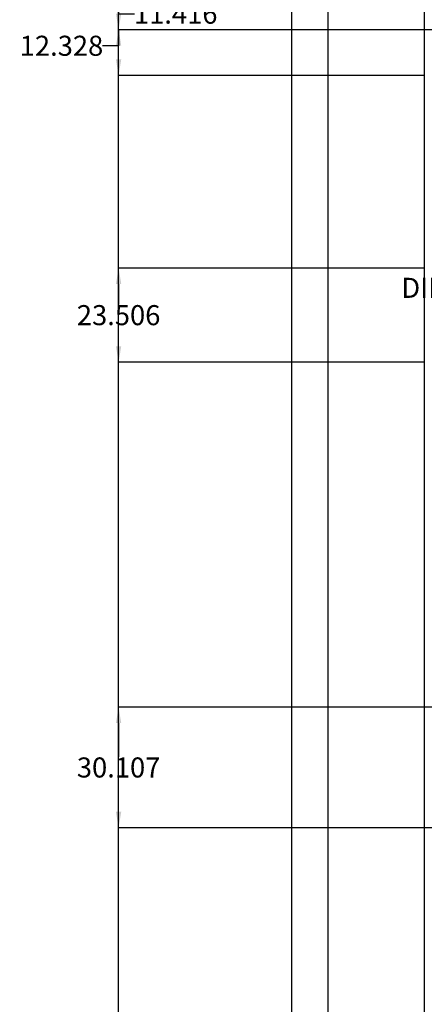
# Model space of a CAD drawing. Units: inches. Extents: x 882 to 1363, y 890 to 1847.
# Tile 2 of 9: x 882 to 983, y 1106 to 1351. Entities that reach past the tile are written whole.
import ezdxf

# ---------------------------------------------------------------- set-up
doc = ezdxf.new("R2010")
doc.units = ezdxf.units.IN
doc.header["$MEASUREMENT"] = 0
doc.layers.add('A-ANNO-DIMS', color=2, linetype='Continuous', lineweight=18)
doc.layers.add('C-PROP', color=7, linetype='Continuous', lineweight=25)
doc.styles.get("Standard").update_dxf_attribs({"font": 'arial.ttf'})
doc.dimstyles.get("Standard").update_dxf_attribs({"dimtxt": 5, "dimasz": 4, "dimexe": 0.18, "dimexo": 0.0625, "dimgap": 0.09, "dimtad": 0, "dimtih": 1, "dimtoh": 1, "dimdec": 1, "dimzin": 0, "dimdsep": 46, "dimlunit": 3, "dimtxsty": 'Standard', "dimcen": 0.09, "dimadec": 0, "dimazin": 0, "dimtfac": 1, "dimtdec": 1, "dimtofl": 0, "dimtmove": 0, "dimatfit": 3, "dimfxl": 1, "dimtolj": 1, "dimtzin": 0, "dimarcsym": 0})

# ---------------------------------------------------------------- blocks, each defined once
blk = doc.blocks.new('*D27')
at = {"layer": 'A-ANNO-DIMS', "color": 0, "lineweight": -2, "transparency": 16777216}
for p, q in [((1013.72, 1329.89), (999.96, 1329.89)), ((1000.14, 1325.89), (1000.14, 1287.07)), ((1000.14, 1242.89), (1000.14, 1281.72)), ((1013.72, 1238.89), (999.96, 1238.89))]:
    blk.add_line(p, q, dxfattribs=at)
at = {"layer": 'A-ANNO-DIMS', "color": 0, "transparency": 16777216}
for points in [[(999.47, 1325.89), (1000.8, 1325.89), (1000.14, 1329.89)], [(999.47, 1242.89), (1000.8, 1242.89), (1000.14, 1238.89)]]:
    blk.add_solid(points, dxfattribs=at)
at = {"layer": 'Defpoints', "color": 0, "transparency": 16777216}
for p in [(1013.79, 1329.89), (1000.14, 1238.89), (1013.79, 1238.89)]:
    blk.add_point(p, dxfattribs=at)
at = {"layer": 'A-ANNO-DIMS', "color": 0, "transparency": 16777216, "insert": (1000.14, 1284.39), "char_height": 5, "attachment_point": 5}
blk.add_mtext('\\A1;DINING SET 91', dxfattribs=at)
blk = doc.blocks.new('*D37')
at = {"layer": 'A-ANNO-DIMS', "color": 0, "lineweight": -2, "transparency": 16777216}
for p, q in [((982.78, 1767.75), (906.46, 1767.75)), ((906.64, 1763.75), (906.64, 1383.34)), ((906.64, 997.75), (906.64, 1378.16)), ((982.78, 993.75), (906.46, 993.75))]:
    blk.add_line(p, q, dxfattribs=at)
at = {"layer": 'A-ANNO-DIMS', "color": 0, "transparency": 16777216}
for points in [[(905.97, 1763.75), (907.3, 1763.75), (906.64, 1767.75)], [(905.97, 997.75), (907.3, 997.75), (906.64, 993.75)]]:
    blk.add_solid(points, dxfattribs=at)
at = {"layer": 'Defpoints', "color": 0, "transparency": 16777216}
for p in [(906.64, 1767.75), (982.84, 1767.75), (982.84, 993.75)]:
    blk.add_point(p, dxfattribs=at)
at = {"layer": 'A-ANNO-DIMS', "color": 0, "transparency": 16777216, "insert": (906.64, 1380.75), "char_height": 5, "attachment_point": 5}
blk.add_mtext('\\A1;774', dxfattribs=at)
blk = doc.blocks.new('*D51')
at = {"layer": 'A-ANNO-DIMS', "color": 0, "lineweight": -2, "transparency": 16777216}
for p, q in [((982.84, 1767.69), (982.84, 893.37)), ((1000.84, 1767.69), (1000.84, 893.37)), ((986.84, 893.55), (996.84, 893.55)), ((1000.84, 893.55), (1004.84, 893.55))]:
    blk.add_line(p, q, dxfattribs=at)
at = {"layer": 'A-ANNO-DIMS', "color": 0, "transparency": 16777216}
for points in [[(986.84, 894.21), (986.84, 892.88), (982.84, 893.55)], [(996.84, 894.21), (996.84, 892.88), (1000.84, 893.55)]]:
    blk.add_solid(points, dxfattribs=at)
at = {"layer": 'Defpoints', "color": 0, "transparency": 16777216}
for p in [(982.84, 1767.75), (1000.84, 1767.75), (1000.84, 893.55)]:
    blk.add_point(p, dxfattribs=at)
at = {"layer": 'A-ANNO-DIMS', "color": 0, "transparency": 16777216, "insert": (1015.08, 893.55), "char_height": 5, "attachment_point": 5}
blk.add_mtext('\\A1;18.006', dxfattribs=at)
blk = doc.blocks.new('*D59')
at = {"layer": 'A-ANNO-DIMS', "color": 0, "lineweight": -2, "transparency": 16777216}
for p, q in [((982.78, 1361.08), (906.46, 1361.08)), ((906.64, 1357.08), (906.64, 1352.75)), ((991.78, 1348.75), (906.46, 1348.75)), ((906.64, 1348.75), (906.64, 1344.75)), ((906.64, 1344.75), (902.64, 1344.75))]:
    blk.add_line(p, q, dxfattribs=at)
at = {"layer": 'A-ANNO-DIMS', "color": 0, "transparency": 16777216}
for points in [[(905.97, 1357.08), (907.3, 1357.08), (906.64, 1361.08)], [(905.97, 1352.75), (907.3, 1352.75), (906.64, 1348.75)]]:
    blk.add_solid(points, dxfattribs=at)
at = {"layer": 'Defpoints', "color": 0, "transparency": 16777216}
for p in [(982.84, 1361.08), (906.64, 1348.75), (991.84, 1348.75)]:
    blk.add_point(p, dxfattribs=at)
at = {"layer": 'A-ANNO-DIMS', "color": 0, "transparency": 16777216, "insert": (892.4, 1344.75), "char_height": 5, "attachment_point": 5}
blk.add_mtext('\\A1;12.328', dxfattribs=at)
blk = doc.blocks.new('*D71')
at = {"layer": 'A-ANNO-DIMS', "color": 0, "lineweight": -2, "transparency": 16777216}
for p, q in [((1243.78, 1179.86), (906.46, 1179.86)), ((906.64, 1175.86), (906.64, 1167.45)), ((906.64, 1153.75), (906.64, 1162.16)), ((1243.78, 1149.75), (906.46, 1149.75))]:
    blk.add_line(p, q, dxfattribs=at)
at = {"layer": 'A-ANNO-DIMS', "color": 0, "transparency": 16777216}
for points in [[(905.97, 1175.86), (907.3, 1175.86), (906.64, 1179.86)], [(905.97, 1153.75), (907.3, 1153.75), (906.64, 1149.75)]]:
    blk.add_solid(points, dxfattribs=at)
at = {"layer": 'Defpoints', "color": 0, "transparency": 16777216}
for p in [(906.64, 1179.86), (1243.84, 1179.86), (1243.84, 1149.75)]:
    blk.add_point(p, dxfattribs=at)
at = {"layer": 'A-ANNO-DIMS', "color": 0, "transparency": 16777216, "insert": (906.64, 1164.8), "char_height": 5, "attachment_point": 5}
blk.add_mtext('\\A1;30.107', dxfattribs=at)
blk = doc.blocks.new('*D79')
at = {"layer": 'A-ANNO-DIMS', "color": 0, "lineweight": -2, "transparency": 16777216}
for p, q in [((982.78, 1289.33), (906.46, 1289.33)), ((906.64, 1285.33), (906.64, 1280.22)), ((906.64, 1269.83), (906.64, 1274.94)), ((982.78, 1265.83), (906.46, 1265.83))]:
    blk.add_line(p, q, dxfattribs=at)
at = {"layer": 'A-ANNO-DIMS', "color": 0, "transparency": 16777216}
for points in [[(905.97, 1285.33), (907.3, 1285.33), (906.64, 1289.33)], [(905.97, 1269.83), (907.3, 1269.83), (906.64, 1265.83)]]:
    blk.add_solid(points, dxfattribs=at)
at = {"layer": 'Defpoints', "color": 0, "transparency": 16777216}
for p in [(906.64, 1289.33), (982.84, 1289.33), (982.84, 1265.83)]:
    blk.add_point(p, dxfattribs=at)
at = {"layer": 'A-ANNO-DIMS', "color": 0, "transparency": 16777216, "insert": (906.64, 1277.58), "char_height": 5, "attachment_point": 5}
blk.add_mtext('\\A1;23.506', dxfattribs=at)
blk = doc.blocks.new('*D83')
at = {"layer": 'A-ANNO-DIMS', "color": 0, "lineweight": -2, "transparency": 16777216}
for p, q in [((906.64, 1348.75), (906.64, 1352.75)), ((906.64, 1352.75), (910.64, 1352.75)), ((991.78, 1348.75), (906.46, 1348.75)), ((906.64, 1341.33), (906.64, 1344.75)), ((982.78, 1337.33), (906.46, 1337.33))]:
    blk.add_line(p, q, dxfattribs=at)
at = {"layer": 'A-ANNO-DIMS', "color": 0, "transparency": 16777216}
for points in [[(905.97, 1344.75), (907.3, 1344.75), (906.64, 1348.75)], [(905.97, 1341.33), (907.3, 1341.33), (906.64, 1337.33)]]:
    blk.add_solid(points, dxfattribs=at)
at = {"layer": 'Defpoints', "color": 0, "transparency": 16777216}
for p in [(906.64, 1348.75), (991.84, 1348.75), (982.84, 1337.33)]:
    blk.add_point(p, dxfattribs=at)
at = {"layer": 'A-ANNO-DIMS', "color": 0, "transparency": 16777216, "insert": (920.87, 1352.75), "char_height": 5, "attachment_point": 5}
blk.add_mtext('\\A1;11.416', dxfattribs=at)

msp = doc.modelspace()

# ---------------------------------------------------------------- linework, layer by layer
at = {"layer": 'C-PROP'}
for points in [[(949.8388, 1800.7495), (1309.8388, 1800.7495), (1309.8388, 936.7495), (949.8388, 936.7495)], [(958.8388, 1791.7495), (1300.8388, 1791.7495), (1300.8388, 945.7495), (958.8388, 945.7495)]]:
    msp.add_lwpolyline(points, close=True, dxfattribs=at)

# ---------------------------------------------------------------- dimensions: what is measured, and where the dimension line sits
at = {"layer": 'A-ANNO-DIMS'}
for base, p1, p2, override, picture, middle in [((906.6353, 1767.7495), (982.8388, 993.7495), (982.8388, 1767.7495), {"dimdec": 0, "dimlfac": 1, "dimrnd": 0, "dimzin": 0, "dimdsep": 46, "dimlunit": 2}, '*D37', (906.6353, 1380.7495)), ((906.6353, 1348.7495), (982.8388, 1361.0778), (991.8388, 1348.7495), {"dimdec": 3, "dimlfac": 1, "dimrnd": 0, "dimzin": 0, "dimdsep": 46, "dimlunit": 2}, '*D59', (892.397, 1344.7495)), ((906.6353, 1348.7495), (982.8388, 1337.3333), (991.8388, 1348.7495), {"dimdec": 3, "dimlfac": 1, "dimrnd": 0, "dimzin": 0, "dimdsep": 46, "dimlunit": 2}, '*D83', (920.8669, 1352.7495)), ((906.6353, 1289.3333), (982.8388, 1265.8272), (982.8388, 1289.3333), {"dimdec": 3, "dimlfac": 1, "dimrnd": 0, "dimzin": 0, "dimdsep": 46, "dimlunit": 2}, '*D79', (906.6353, 1277.5802)), ((906.6353, 1179.8561), (1243.8388, 1149.7495), (1243.8388, 1179.8561), {"dimdec": 3, "dimlfac": 1, "dimrnd": 0, "dimzin": 0, "dimdsep": 46, "dimlunit": 2}, '*D71', (906.6353, 1164.8028))]:
    dim = msp.add_linear_dim(base=base, p1=p1, p2=p2, angle=90, dimstyle='Standard', override=override, dxfattribs=at)
    dim.commit()
    dim.dimension.update_dxf_attribs({"geometry": picture, "text_midpoint": middle})
dim = msp.add_linear_dim(base=(1000.8447, 893.546), p1=(982.8388, 1767.7495), p2=(1000.8447, 1767.7495), dimstyle='Standard', override={"dimdec": 3, "dimlfac": 1, "dimrnd": 0, "dimzin": 0, "dimdsep": 46, "dimlunit": 2}, dxfattribs=at)
dim.commit()
dim.dimension.update_dxf_attribs({"geometry": '*D51', "text_midpoint": (1015.0762, 893.546)})
dim = msp.add_linear_dim(base=(1000.1374, 1238.8919), p1=(1013.7874, 1329.8919), p2=(1013.7874, 1238.8919), angle=270, text='DINING SET <>', dimstyle='Standard', override={"dimdec": 0, "dimlfac": 1, "dimrnd": 0, "dimzin": 0, "dimdsep": 46, "dimlunit": 2}, dxfattribs=at)
dim.commit()
dim.dimension.update_dxf_attribs({"geometry": '*D27', "text_midpoint": (1000.1374, 1284.3919)})

doc.saveas('drawing.dxf')
